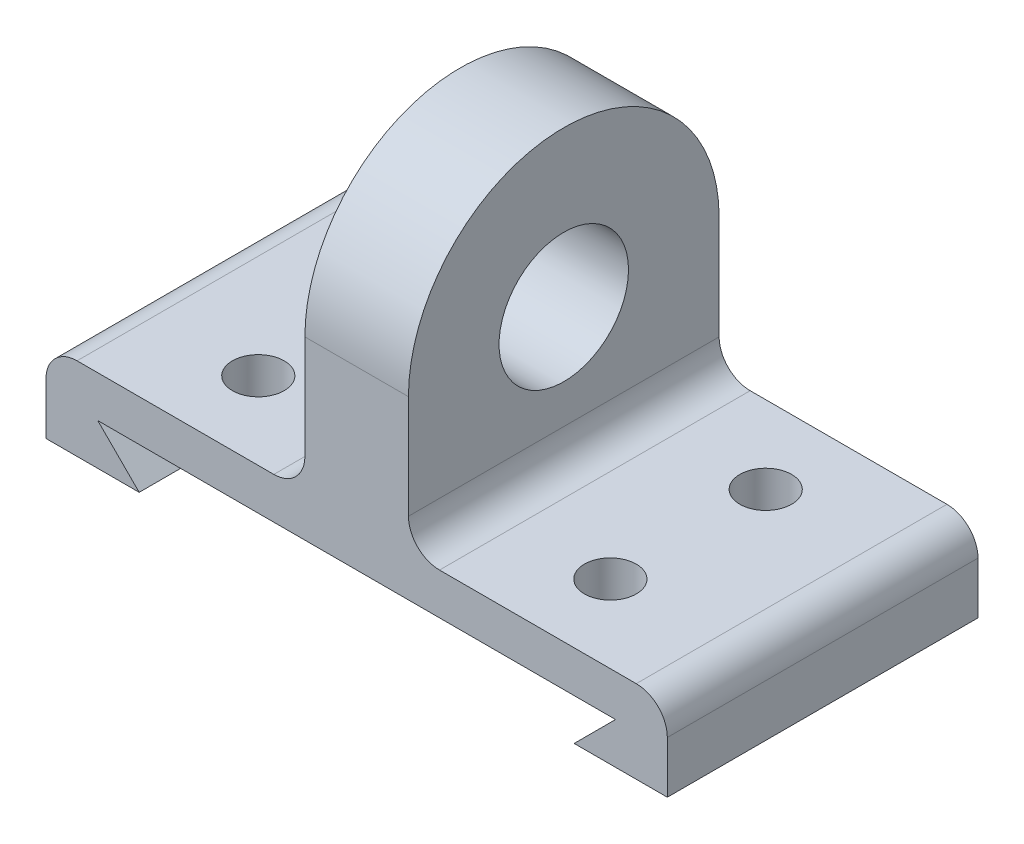
ISO-10303-21;
HEADER;
FILE_DESCRIPTION(('STEP AP214'),'2;1');
FILE_NAME('part.step','',(''),(''),'','','');
FILE_SCHEMA(('AUTOMOTIVE_DESIGN { 1 0 10303 214 1 1 1 1 }'));
ENDSEC;
DATA;
#1=APPLICATION_CONTEXT('core data for automotive mechanical design processes');
#2=APPLICATION_PROTOCOL_DEFINITION('international standard','automotive_design',2000,#1);
#3=PRODUCT_CONTEXT('',#1,'mechanical');
#4=PRODUCT('Part','Part','',(#3));
#5=PRODUCT_RELATED_PRODUCT_CATEGORY('part','',(#4));
#6=PRODUCT_DEFINITION_FORMATION('','',#4);
#7=PRODUCT_DEFINITION_CONTEXT('part definition',#1,'design');
#8=PRODUCT_DEFINITION('design','',#6,#7);
#9=PRODUCT_DEFINITION_SHAPE('','',#8);
#10=(LENGTH_UNIT() NAMED_UNIT(*) SI_UNIT(.MILLI.,.METRE.));
#11=(NAMED_UNIT(*) PLANE_ANGLE_UNIT() SI_UNIT($,.RADIAN.));
#12=(NAMED_UNIT(*) SI_UNIT($,.STERADIAN.) SOLID_ANGLE_UNIT());
#13=UNCERTAINTY_MEASURE_WITH_UNIT(LENGTH_MEASURE(1.E-05),#10,'distance_accuracy_value','');
#14=(GEOMETRIC_REPRESENTATION_CONTEXT(3) GLOBAL_UNCERTAINTY_ASSIGNED_CONTEXT((#13)) GLOBAL_UNIT_ASSIGNED_CONTEXT((#10,
#11,#12)) REPRESENTATION_CONTEXT('',''));
#15=CARTESIAN_POINT('',(0.,0.,0.));
#16=DIRECTION('',(0.,0.,1.));
#17=DIRECTION('',(1.,0.,0.));
#18=AXIS2_PLACEMENT_3D('',#15,#16,#17);
#19=CARTESIAN_POINT('',(60.,8.0000000000001,-60.));
#20=DIRECTION('',(0.,1.,0.));
#21=DIRECTION('',(-1.,0.,0.));
#22=AXIS2_PLACEMENT_3D('',#19,#20,#21);
#23=PLANE('',#22);
#24=CARTESIAN_POINT('',(-34.,8.00000000000009,-15.));
#25=DIRECTION('',(0.,1.,0.));
#26=DIRECTION('',(-1.,0.,0.));
#27=AXIS2_PLACEMENT_3D('',#24,#25,#26);
#28=CIRCLE('',#27,5.);
#29=CARTESIAN_POINT('',(-39.,8.00000000000009,-15.));
#30=VERTEX_POINT('',#29);
#31=EDGE_CURVE('E168',#30,#30,#28,.T.);
#32=ORIENTED_EDGE('',*,*,#31,.F.);
#33=EDGE_LOOP('',(#32));
#34=FACE_BOUND('',#33,.T.);
#35=CARTESIAN_POINT('',(-34.,8.00000000000009,-45.));
#36=DIRECTION('',(0.,1.,0.));
#37=DIRECTION('',(-1.,0.,0.));
#38=AXIS2_PLACEMENT_3D('',#35,#36,#37);
#39=CIRCLE('',#38,5.);
#40=CARTESIAN_POINT('',(-39.,8.00000000000009,-45.));
#41=VERTEX_POINT('',#40);
#42=EDGE_CURVE('E186',#41,#41,#39,.T.);
#43=ORIENTED_EDGE('',*,*,#42,.F.);
#44=EDGE_LOOP('',(#43));
#45=FACE_BOUND('',#44,.T.);
#46=DIRECTION('',(-1.,0.,0.));
#47=VECTOR('',#46,1.);
#48=CARTESIAN_POINT('',(60.,8.0000000000001,-60.));
#49=LINE('',#48,#47);
#50=CARTESIAN_POINT('',(-16.,8.00000000000009,-60.));
#51=VERTEX_POINT('',#50);
#52=CARTESIAN_POINT('',(-54.,8.00000000000008,-60.));
#53=VERTEX_POINT('',#52);
#54=EDGE_CURVE('E211',#51,#53,#49,.T.);
#55=ORIENTED_EDGE('',*,*,#54,.T.);
#56=DIRECTION('',(0.,0.,1.));
#57=VECTOR('',#56,1.);
#58=CARTESIAN_POINT('',(-54.,8.00000000000008,-60.));
#59=LINE('',#58,#57);
#60=CARTESIAN_POINT('',(-54.,8.00000000000008,0.));
#61=VERTEX_POINT('',#60);
#62=EDGE_CURVE('E272',#53,#61,#59,.T.);
#63=ORIENTED_EDGE('',*,*,#62,.T.);
#64=DIRECTION('',(-1.,0.,0.));
#65=VECTOR('',#64,1.);
#66=CARTESIAN_POINT('',(60.,8.0000000000001,0.));
#67=LINE('',#66,#65);
#68=CARTESIAN_POINT('',(-16.,8.00000000000009,0.));
#69=VERTEX_POINT('',#68);
#70=EDGE_CURVE('E237',#69,#61,#67,.T.);
#71=ORIENTED_EDGE('',*,*,#70,.F.);
#72=DIRECTION('',(0.,0.,-1.));
#73=VECTOR('',#72,1.);
#74=CARTESIAN_POINT('',(-16.,8.00000000000009,-60.));
#75=LINE('',#74,#73);
#76=EDGE_CURVE('E247',#69,#51,#75,.T.);
#77=ORIENTED_EDGE('',*,*,#76,.T.);
#78=EDGE_LOOP('',(#55,#63,#71,#77));
#79=FACE_BOUND('',#78,.T.);
#80=ADVANCED_FACE('F39',(#34,#45,#79),#23,.T.);
#81=CARTESIAN_POINT('',(-42.,-7.99999999999992,-60.));
#82=DIRECTION('',(0.707106781186544,0.707106781186551,0.));
#83=DIRECTION('',(-0.707106781186551,0.707106781186544,0.));
#84=AXIS2_PLACEMENT_3D('',#81,#82,#83);
#85=PLANE('',#84);
#86=DIRECTION('',(-0.707106781186551,0.707106781186544,0.));
#87=VECTOR('',#86,1.);
#88=CARTESIAN_POINT('',(-42.,-7.99999999999992,0.));
#89=LINE('',#88,#87);
#90=CARTESIAN_POINT('',(-42.,-7.99999999999992,0.));
#91=VERTEX_POINT('',#90);
#92=CARTESIAN_POINT('',(-50.,0.,0.));
#93=VERTEX_POINT('',#92);
#94=EDGE_CURVE('E201',#91,#93,#89,.T.);
#95=ORIENTED_EDGE('',*,*,#94,.F.);
#96=DIRECTION('',(0.,0.,1.));
#97=VECTOR('',#96,1.);
#98=CARTESIAN_POINT('',(-42.,-7.99999999999992,-60.));
#99=LINE('',#98,#97);
#100=CARTESIAN_POINT('',(-42.,-7.99999999999992,-60.));
#101=VERTEX_POINT('',#100);
#102=EDGE_CURVE('E253',#101,#91,#99,.T.);
#103=ORIENTED_EDGE('',*,*,#102,.F.);
#104=DIRECTION('',(-0.707106781186551,0.707106781186544,0.));
#105=VECTOR('',#104,1.);
#106=CARTESIAN_POINT('',(-42.,-7.99999999999992,-60.));
#107=LINE('',#106,#105);
#108=CARTESIAN_POINT('',(-50.,0.,-60.));
#109=VERTEX_POINT('',#108);
#110=EDGE_CURVE('E218',#101,#109,#107,.T.);
#111=ORIENTED_EDGE('',*,*,#110,.T.);
#112=DIRECTION('',(0.,0.,1.));
#113=VECTOR('',#112,1.);
#114=CARTESIAN_POINT('',(-50.,0.,-60.));
#115=LINE('',#114,#113);
#116=EDGE_CURVE('E246',#109,#93,#115,.T.);
#117=ORIENTED_EDGE('',*,*,#116,.T.);
#118=EDGE_LOOP('',(#95,#103,#111,#117));
#119=FACE_BOUND('',#118,.T.);
#120=ADVANCED_FACE('F343',(#119),#85,.T.);
#121=CARTESIAN_POINT('',(-60.,-7.99999999999992,-60.));
#122=DIRECTION('',(0.,-1.,0.));
#123=DIRECTION('',(0.,0.,-1.));
#124=AXIS2_PLACEMENT_3D('',#121,#122,#123);
#125=PLANE('',#124);
#126=DIRECTION('',(1.,0.,0.));
#127=VECTOR('',#126,1.);
#128=CARTESIAN_POINT('',(-60.,-7.99999999999992,0.));
#129=LINE('',#128,#127);
#130=CARTESIAN_POINT('',(-60.,-7.99999999999992,0.));
#131=VERTEX_POINT('',#130);
#132=EDGE_CURVE('E244',#131,#91,#129,.T.);
#133=ORIENTED_EDGE('',*,*,#132,.F.);
#134=DIRECTION('',(0.,0.,1.));
#135=VECTOR('',#134,1.);
#136=CARTESIAN_POINT('',(-60.,-7.99999999999992,-60.));
#137=LINE('',#136,#135);
#138=CARTESIAN_POINT('',(-60.,-7.99999999999992,-60.));
#139=VERTEX_POINT('',#138);
#140=EDGE_CURVE('E251',#139,#131,#137,.T.);
#141=ORIENTED_EDGE('',*,*,#140,.F.);
#142=DIRECTION('',(1.,0.,0.));
#143=VECTOR('',#142,1.);
#144=CARTESIAN_POINT('',(-60.,-7.99999999999992,-60.));
#145=LINE('',#144,#143);
#146=EDGE_CURVE('E216',#139,#101,#145,.T.);
#147=ORIENTED_EDGE('',*,*,#146,.T.);
#148=ORIENTED_EDGE('',*,*,#102,.T.);
#149=EDGE_LOOP('',(#133,#141,#147,#148));
#150=FACE_BOUND('',#149,.T.);
#151=ADVANCED_FACE('F346',(#150),#125,.T.);
#152=CARTESIAN_POINT('',(-60.,8.00000000000008,-60.));
#153=DIRECTION('',(-1.,0.,0.));
#154=DIRECTION('',(0.,0.,1.));
#155=AXIS2_PLACEMENT_3D('',#152,#153,#154);
#156=PLANE('',#155);
#157=DIRECTION('',(0.,-1.,0.));
#158=VECTOR('',#157,1.);
#159=CARTESIAN_POINT('',(-60.,8.00000000000008,0.));
#160=LINE('',#159,#158);
#161=CARTESIAN_POINT('',(-60.,2.00000000000008,0.));
#162=VERTEX_POINT('',#161);
#163=EDGE_CURVE('E238',#162,#131,#160,.T.);
#164=ORIENTED_EDGE('',*,*,#163,.F.);
#165=DIRECTION('',(0.,0.,1.));
#166=VECTOR('',#165,1.);
#167=CARTESIAN_POINT('',(-60.,2.00000000000008,-60.));
#168=LINE('',#167,#166);
#169=CARTESIAN_POINT('',(-60.,2.00000000000008,-60.));
#170=VERTEX_POINT('',#169);
#171=EDGE_CURVE('E278',#162,#170,#168,.F.);
#172=ORIENTED_EDGE('',*,*,#171,.T.);
#173=DIRECTION('',(0.,-1.,0.));
#174=VECTOR('',#173,1.);
#175=CARTESIAN_POINT('',(-60.,8.00000000000008,-60.));
#176=LINE('',#175,#174);
#177=EDGE_CURVE('E212',#170,#139,#176,.T.);
#178=ORIENTED_EDGE('',*,*,#177,.T.);
#179=ORIENTED_EDGE('',*,*,#140,.T.);
#180=EDGE_LOOP('',(#164,#172,#178,#179));
#181=FACE_BOUND('',#180,.T.);
#182=ADVANCED_FACE('F351',(#181),#156,.T.);
#183=CARTESIAN_POINT('',(54.,8.0000000000001,-60.));
#184=VERTEX_POINT('',#183);
#185=CARTESIAN_POINT('',(16.,8.00000000000009,-60.));
#186=VERTEX_POINT('',#185);
#187=EDGE_CURVE('E215',#184,#186,#49,.T.);
#188=ORIENTED_EDGE('',*,*,#187,.T.);
#189=DIRECTION('',(0.,0.,-1.));
#190=VECTOR('',#189,1.);
#191=CARTESIAN_POINT('',(16.,8.00000000000009,0.));
#192=LINE('',#191,#190);
#193=CARTESIAN_POINT('',(16.,8.00000000000009,0.));
#194=VERTEX_POINT('',#193);
#195=EDGE_CURVE('E287',#186,#194,#192,.F.);
#196=ORIENTED_EDGE('',*,*,#195,.T.);
#197=CARTESIAN_POINT('',(54.,8.0000000000001,0.));
#198=VERTEX_POINT('',#197);
#199=EDGE_CURVE('E240',#198,#194,#67,.T.);
#200=ORIENTED_EDGE('',*,*,#199,.F.);
#201=DIRECTION('',(0.,0.,1.));
#202=VECTOR('',#201,1.);
#203=CARTESIAN_POINT('',(54.,8.0000000000001,-60.));
#204=LINE('',#203,#202);
#205=EDGE_CURVE('E290',#198,#184,#204,.F.);
#206=ORIENTED_EDGE('',*,*,#205,.T.);
#207=EDGE_LOOP('',(#188,#196,#200,#206));
#208=FACE_BOUND('',#207,.T.);
#209=CARTESIAN_POINT('',(34.,8.00000000000009,-15.));
#210=DIRECTION('',(0.,1.,0.));
#211=DIRECTION('',(-1.,0.,0.));
#212=AXIS2_PLACEMENT_3D('',#209,#210,#211);
#213=CIRCLE('',#212,5.);
#214=CARTESIAN_POINT('',(29.,8.00000000000009,-15.));
#215=VERTEX_POINT('',#214);
#216=EDGE_CURVE('E194',#215,#215,#213,.T.);
#217=ORIENTED_EDGE('',*,*,#216,.F.);
#218=EDGE_LOOP('',(#217));
#219=FACE_BOUND('',#218,.T.);
#220=CARTESIAN_POINT('',(34.,8.00000000000009,-45.));
#221=DIRECTION('',(0.,1.,0.));
#222=DIRECTION('',(-1.,0.,0.));
#223=AXIS2_PLACEMENT_3D('',#220,#221,#222);
#224=CIRCLE('',#223,5.);
#225=CARTESIAN_POINT('',(29.,8.00000000000009,-45.));
#226=VERTEX_POINT('',#225);
#227=EDGE_CURVE('E193',#226,#226,#224,.T.);
#228=ORIENTED_EDGE('',*,*,#227,.F.);
#229=EDGE_LOOP('',(#228));
#230=FACE_BOUND('',#229,.T.);
#231=ADVANCED_FACE('F321',(#208,#219,#230),#23,.T.);
#232=CARTESIAN_POINT('',(60.,-7.99999999999991,-60.));
#233=DIRECTION('',(1.,0.,0.));
#234=DIRECTION('',(0.,0.,-1.));
#235=AXIS2_PLACEMENT_3D('',#232,#233,#234);
#236=PLANE('',#235);
#237=DIRECTION('',(0.,1.,0.));
#238=VECTOR('',#237,1.);
#239=CARTESIAN_POINT('',(60.,-7.99999999999991,-60.));
#240=LINE('',#239,#238);
#241=CARTESIAN_POINT('',(60.,-7.99999999999991,-60.));
#242=VERTEX_POINT('',#241);
#243=CARTESIAN_POINT('',(60.,2.0000000000001,-60.));
#244=VERTEX_POINT('',#243);
#245=EDGE_CURVE('E207',#242,#244,#240,.T.);
#246=ORIENTED_EDGE('',*,*,#245,.T.);
#247=DIRECTION('',(0.,0.,1.));
#248=VECTOR('',#247,1.);
#249=CARTESIAN_POINT('',(60.,2.0000000000001,-60.));
#250=LINE('',#249,#248);
#251=CARTESIAN_POINT('',(60.,2.0000000000001,0.));
#252=VERTEX_POINT('',#251);
#253=EDGE_CURVE('E295',#244,#252,#250,.T.);
#254=ORIENTED_EDGE('',*,*,#253,.T.);
#255=DIRECTION('',(0.,1.,0.));
#256=VECTOR('',#255,1.);
#257=CARTESIAN_POINT('',(60.,-7.99999999999991,0.));
#258=LINE('',#257,#256);
#259=CARTESIAN_POINT('',(60.,-7.99999999999991,0.));
#260=VERTEX_POINT('',#259);
#261=EDGE_CURVE('E235',#260,#252,#258,.T.);
#262=ORIENTED_EDGE('',*,*,#261,.F.);
#263=DIRECTION('',(0.,0.,1.));
#264=VECTOR('',#263,1.);
#265=CARTESIAN_POINT('',(60.,-7.99999999999991,-60.));
#266=LINE('',#265,#264);
#267=EDGE_CURVE('E258',#242,#260,#266,.T.);
#268=ORIENTED_EDGE('',*,*,#267,.F.);
#269=EDGE_LOOP('',(#246,#254,#262,#268));
#270=FACE_BOUND('',#269,.T.);
#271=ADVANCED_FACE('F327',(#270),#236,.T.);
#272=CARTESIAN_POINT('',(42.,-7.99999999999991,-60.));
#273=DIRECTION('',(0.,-1.,0.));
#274=DIRECTION('',(0.,0.,-1.));
#275=AXIS2_PLACEMENT_3D('',#272,#273,#274);
#276=PLANE('',#275);
#277=DIRECTION('',(1.,0.,0.));
#278=VECTOR('',#277,1.);
#279=CARTESIAN_POINT('',(42.,-7.99999999999991,0.));
#280=LINE('',#279,#278);
#281=CARTESIAN_POINT('',(42.,-7.99999999999991,0.));
#282=VERTEX_POINT('',#281);
#283=EDGE_CURVE('E226',#282,#260,#280,.T.);
#284=ORIENTED_EDGE('',*,*,#283,.F.);
#285=DIRECTION('',(0.,0.,1.));
#286=VECTOR('',#285,1.);
#287=CARTESIAN_POINT('',(42.,-7.99999999999991,-60.));
#288=LINE('',#287,#286);
#289=CARTESIAN_POINT('',(42.,-7.99999999999991,-60.));
#290=VERTEX_POINT('',#289);
#291=EDGE_CURVE('E256',#290,#282,#288,.T.);
#292=ORIENTED_EDGE('',*,*,#291,.F.);
#293=DIRECTION('',(1.,0.,0.));
#294=VECTOR('',#293,1.);
#295=CARTESIAN_POINT('',(42.,-7.99999999999991,-60.));
#296=LINE('',#295,#294);
#297=EDGE_CURVE('E206',#290,#242,#296,.T.);
#298=ORIENTED_EDGE('',*,*,#297,.T.);
#299=ORIENTED_EDGE('',*,*,#267,.T.);
#300=EDGE_LOOP('',(#284,#292,#298,#299));
#301=FACE_BOUND('',#300,.T.);
#302=ADVANCED_FACE('F334',(#301),#276,.T.);
#303=CARTESIAN_POINT('',(50.,0.,-60.));
#304=DIRECTION('',(-0.707106781186544,0.707106781186551,0.));
#305=DIRECTION('',(-0.707106781186551,-0.707106781186544,0.));
#306=AXIS2_PLACEMENT_3D('',#303,#304,#305);
#307=PLANE('',#306);
#308=DIRECTION('',(-0.707106781186551,-0.707106781186544,0.));
#309=VECTOR('',#308,1.);
#310=CARTESIAN_POINT('',(50.,0.,0.));
#311=LINE('',#310,#309);
#312=CARTESIAN_POINT('',(50.,0.,0.));
#313=VERTEX_POINT('',#312);
#314=EDGE_CURVE('E228',#313,#282,#311,.T.);
#315=ORIENTED_EDGE('',*,*,#314,.F.);
#316=DIRECTION('',(0.,0.,1.));
#317=VECTOR('',#316,1.);
#318=CARTESIAN_POINT('',(50.,0.,-60.));
#319=LINE('',#318,#317);
#320=CARTESIAN_POINT('',(50.,0.,-60.));
#321=VERTEX_POINT('',#320);
#322=EDGE_CURVE('E225',#321,#313,#319,.T.);
#323=ORIENTED_EDGE('',*,*,#322,.F.);
#324=DIRECTION('',(-0.707106781186551,-0.707106781186544,0.));
#325=VECTOR('',#324,1.);
#326=CARTESIAN_POINT('',(50.,0.,-60.));
#327=LINE('',#326,#325);
#328=EDGE_CURVE('E205',#321,#290,#327,.T.);
#329=ORIENTED_EDGE('',*,*,#328,.T.);
#330=ORIENTED_EDGE('',*,*,#291,.T.);
#331=EDGE_LOOP('',(#315,#323,#329,#330));
#332=FACE_BOUND('',#331,.T.);
#333=ADVANCED_FACE('F338',(#332),#307,.T.);
#334=CARTESIAN_POINT('',(0.,0.,-60.));
#335=DIRECTION('',(0.,-1.,0.));
#336=DIRECTION('',(0.,0.,-1.));
#337=AXIS2_PLACEMENT_3D('',#334,#335,#336);
#338=PLANE('',#337);
#339=CARTESIAN_POINT('',(34.,0.,-15.));
#340=DIRECTION('',(0.,-1.,0.));
#341=DIRECTION('',(0.,0.,-1.));
#342=AXIS2_PLACEMENT_3D('',#339,#340,#341);
#343=CIRCLE('',#342,5.);
#344=CARTESIAN_POINT('',(34.,0.,-20.));
#345=VERTEX_POINT('',#344);
#346=EDGE_CURVE('E229',#345,#345,#343,.T.);
#347=ORIENTED_EDGE('',*,*,#346,.F.);
#348=EDGE_LOOP('',(#347));
#349=FACE_BOUND('',#348,.T.);
#350=CARTESIAN_POINT('',(-34.,0.,-45.));
#351=DIRECTION('',(0.,-1.,0.));
#352=DIRECTION('',(0.,0.,-1.));
#353=AXIS2_PLACEMENT_3D('',#350,#351,#352);
#354=CIRCLE('',#353,5.);
#355=CARTESIAN_POINT('',(-34.,0.,-50.));
#356=VERTEX_POINT('',#355);
#357=EDGE_CURVE('E266',#356,#356,#354,.T.);
#358=ORIENTED_EDGE('',*,*,#357,.F.);
#359=EDGE_LOOP('',(#358));
#360=FACE_BOUND('',#359,.T.);
#361=CARTESIAN_POINT('',(-34.,0.,-15.));
#362=DIRECTION('',(0.,-1.,0.));
#363=DIRECTION('',(0.,0.,-1.));
#364=AXIS2_PLACEMENT_3D('',#361,#362,#363);
#365=CIRCLE('',#364,5.);
#366=CARTESIAN_POINT('',(-34.,0.,-20.));
#367=VERTEX_POINT('',#366);
#368=EDGE_CURVE('E263',#367,#367,#365,.T.);
#369=ORIENTED_EDGE('',*,*,#368,.F.);
#370=EDGE_LOOP('',(#369));
#371=FACE_BOUND('',#370,.T.);
#372=CARTESIAN_POINT('',(34.,0.,-45.));
#373=DIRECTION('',(0.,-1.,0.));
#374=DIRECTION('',(0.,0.,-1.));
#375=AXIS2_PLACEMENT_3D('',#372,#373,#374);
#376=CIRCLE('',#375,5.);
#377=CARTESIAN_POINT('',(34.,0.,-50.));
#378=VERTEX_POINT('',#377);
#379=EDGE_CURVE('E200',#378,#378,#376,.T.);
#380=ORIENTED_EDGE('',*,*,#379,.F.);
#381=EDGE_LOOP('',(#380));
#382=FACE_BOUND('',#381,.T.);
#383=DIRECTION('',(1.,0.,0.));
#384=VECTOR('',#383,1.);
#385=CARTESIAN_POINT('',(0.,0.,0.));
#386=LINE('',#385,#384);
#387=EDGE_CURVE('E224',#93,#313,#386,.T.);
#388=ORIENTED_EDGE('',*,*,#387,.F.);
#389=ORIENTED_EDGE('',*,*,#116,.F.);
#390=DIRECTION('',(1.,0.,0.));
#391=VECTOR('',#390,1.);
#392=CARTESIAN_POINT('',(-50.,0.,-60.));
#393=LINE('',#392,#391);
#394=EDGE_CURVE('E199',#109,#321,#393,.T.);
#395=ORIENTED_EDGE('',*,*,#394,.T.);
#396=ORIENTED_EDGE('',*,*,#322,.T.);
#397=EDGE_LOOP('',(#388,#389,#395,#396));
#398=FACE_BOUND('',#397,.T.);
#399=ADVANCED_FACE('F359',(#349,#360,#371,#382,#398),#338,.T.);
#400=CARTESIAN_POINT('',(0.,0.,-60.));
#401=DIRECTION('',(0.,0.,1.));
#402=DIRECTION('',(1.,0.,0.));
#403=AXIS2_PLACEMENT_3D('',#400,#401,#402);
#404=PLANE('',#403);
#405=ORIENTED_EDGE('',*,*,#177,.F.);
#406=CARTESIAN_POINT('',(-54.,2.00000000000008,-60.));
#407=DIRECTION('',(0.,0.,1.));
#408=DIRECTION('',(1.,0.,0.));
#409=AXIS2_PLACEMENT_3D('',#406,#407,#408);
#410=CIRCLE('',#409,6.);
#411=EDGE_CURVE('E282',#170,#53,#410,.F.);
#412=ORIENTED_EDGE('',*,*,#411,.T.);
#413=ORIENTED_EDGE('',*,*,#54,.F.);
#414=CARTESIAN_POINT('',(-16.,14.0000000000001,-60.));
#415=DIRECTION('',(0.,0.,1.));
#416=DIRECTION('',(1.,0.,0.));
#417=AXIS2_PLACEMENT_3D('',#414,#415,#416);
#418=CIRCLE('',#417,6.);
#419=CARTESIAN_POINT('',(-10.,14.0000000000001,-60.));
#420=VERTEX_POINT('',#419);
#421=EDGE_CURVE('E293',#51,#420,#418,.T.);
#422=ORIENTED_EDGE('',*,*,#421,.T.);
#423=DIRECTION('',(0.,1.,0.));
#424=VECTOR('',#423,1.);
#425=CARTESIAN_POINT('',(-10.,8.0000000000001,-60.));
#426=LINE('',#425,#424);
#427=CARTESIAN_POINT('',(-10.,34.0000000000001,-60.));
#428=VERTEX_POINT('',#427);
#429=EDGE_CURVE('E170',#420,#428,#426,.T.);
#430=ORIENTED_EDGE('',*,*,#429,.T.);
#431=DIRECTION('',(-1.,0.,0.));
#432=VECTOR('',#431,1.);
#433=CARTESIAN_POINT('',(10.,34.0000000000001,-60.));
#434=LINE('',#433,#432);
#435=CARTESIAN_POINT('',(10.,34.0000000000001,-60.));
#436=VERTEX_POINT('',#435);
#437=EDGE_CURVE('E162',#436,#428,#434,.T.);
#438=ORIENTED_EDGE('',*,*,#437,.F.);
#439=DIRECTION('',(0.,1.,0.));
#440=VECTOR('',#439,1.);
#441=CARTESIAN_POINT('',(10.,8.0000000000001,-60.));
#442=LINE('',#441,#440);
#443=CARTESIAN_POINT('',(10.,14.0000000000001,-60.));
#444=VERTEX_POINT('',#443);
#445=EDGE_CURVE('E147',#444,#436,#442,.T.);
#446=ORIENTED_EDGE('',*,*,#445,.F.);
#447=CARTESIAN_POINT('',(16.,14.0000000000001,-60.));
#448=DIRECTION('',(0.,0.,1.));
#449=DIRECTION('',(1.,0.,0.));
#450=AXIS2_PLACEMENT_3D('',#447,#448,#449);
#451=CIRCLE('',#450,6.);
#452=EDGE_CURVE('E50',#444,#186,#451,.T.);
#453=ORIENTED_EDGE('',*,*,#452,.T.);
#454=ORIENTED_EDGE('',*,*,#187,.F.);
#455=CARTESIAN_POINT('',(54.,2.0000000000001,-60.));
#456=DIRECTION('',(0.,0.,1.));
#457=DIRECTION('',(1.,0.,0.));
#458=AXIS2_PLACEMENT_3D('',#455,#456,#457);
#459=CIRCLE('',#458,6.);
#460=EDGE_CURVE('E53',#184,#244,#459,.F.);
#461=ORIENTED_EDGE('',*,*,#460,.T.);
#462=ORIENTED_EDGE('',*,*,#245,.F.);
#463=ORIENTED_EDGE('',*,*,#297,.F.);
#464=ORIENTED_EDGE('',*,*,#328,.F.);
#465=ORIENTED_EDGE('',*,*,#394,.F.);
#466=ORIENTED_EDGE('',*,*,#110,.F.);
#467=ORIENTED_EDGE('',*,*,#146,.F.);
#468=EDGE_LOOP('',(#405,#412,#413,#422,#430,#438,#446,#453,#454,#461,#462,#463,#464,#465,#466,#467));
#469=FACE_BOUND('',#468,.T.);
#470=ADVANCED_FACE('F164',(#469),#404,.F.);
#471=CARTESIAN_POINT('',(0.,0.,0.));
#472=DIRECTION('',(0.,0.,1.));
#473=DIRECTION('',(1.,0.,0.));
#474=AXIS2_PLACEMENT_3D('',#471,#472,#473);
#475=PLANE('',#474);
#476=ORIENTED_EDGE('',*,*,#70,.T.);
#477=CARTESIAN_POINT('',(-54.,2.00000000000008,0.));
#478=DIRECTION('',(0.,0.,1.));
#479=DIRECTION('',(1.,0.,0.));
#480=AXIS2_PLACEMENT_3D('',#477,#478,#479);
#481=CIRCLE('',#480,6.);
#482=EDGE_CURVE('E279',#61,#162,#481,.T.);
#483=ORIENTED_EDGE('',*,*,#482,.T.);
#484=ORIENTED_EDGE('',*,*,#163,.T.);
#485=ORIENTED_EDGE('',*,*,#132,.T.);
#486=ORIENTED_EDGE('',*,*,#94,.T.);
#487=ORIENTED_EDGE('',*,*,#387,.T.);
#488=ORIENTED_EDGE('',*,*,#314,.T.);
#489=ORIENTED_EDGE('',*,*,#283,.T.);
#490=ORIENTED_EDGE('',*,*,#261,.T.);
#491=CARTESIAN_POINT('',(54.,2.0000000000001,0.));
#492=DIRECTION('',(0.,0.,1.));
#493=DIRECTION('',(1.,0.,0.));
#494=AXIS2_PLACEMENT_3D('',#491,#492,#493);
#495=CIRCLE('',#494,6.);
#496=EDGE_CURVE('E277',#252,#198,#495,.T.);
#497=ORIENTED_EDGE('',*,*,#496,.T.);
#498=ORIENTED_EDGE('',*,*,#199,.T.);
#499=CARTESIAN_POINT('',(16.,14.0000000000001,0.));
#500=DIRECTION('',(0.,0.,1.));
#501=DIRECTION('',(1.,0.,0.));
#502=AXIS2_PLACEMENT_3D('',#499,#500,#501);
#503=CIRCLE('',#502,6.);
#504=CARTESIAN_POINT('',(10.,14.0000000000001,0.));
#505=VERTEX_POINT('',#504);
#506=EDGE_CURVE('E11',#194,#505,#503,.F.);
#507=ORIENTED_EDGE('',*,*,#506,.T.);
#508=DIRECTION('',(0.,-1.,0.));
#509=VECTOR('',#508,1.);
#510=CARTESIAN_POINT('',(10.,8.0000000000001,0.));
#511=LINE('',#510,#509);
#512=CARTESIAN_POINT('',(10.,34.0000000000001,0.));
#513=VERTEX_POINT('',#512);
#514=EDGE_CURVE('E179',#513,#505,#511,.T.);
#515=ORIENTED_EDGE('',*,*,#514,.F.);
#516=DIRECTION('',(-1.,0.,0.));
#517=VECTOR('',#516,1.);
#518=CARTESIAN_POINT('',(10.,34.0000000000001,0.));
#519=LINE('',#518,#517);
#520=CARTESIAN_POINT('',(-10.,34.0000000000001,0.));
#521=VERTEX_POINT('',#520);
#522=EDGE_CURVE('E173',#513,#521,#519,.T.);
#523=ORIENTED_EDGE('',*,*,#522,.T.);
#524=DIRECTION('',(0.,-1.,0.));
#525=VECTOR('',#524,1.);
#526=CARTESIAN_POINT('',(-10.,8.0000000000001,0.));
#527=LINE('',#526,#525);
#528=CARTESIAN_POINT('',(-10.,14.0000000000001,0.));
#529=VERTEX_POINT('',#528);
#530=EDGE_CURVE('E159',#521,#529,#527,.T.);
#531=ORIENTED_EDGE('',*,*,#530,.T.);
#532=CARTESIAN_POINT('',(-16.,14.0000000000001,0.));
#533=DIRECTION('',(0.,0.,1.));
#534=DIRECTION('',(1.,0.,0.));
#535=AXIS2_PLACEMENT_3D('',#532,#533,#534);
#536=CIRCLE('',#535,6.);
#537=EDGE_CURVE('E299',#529,#69,#536,.F.);
#538=ORIENTED_EDGE('',*,*,#537,.T.);
#539=EDGE_LOOP('',(#476,#483,#484,#485,#486,#487,#488,#489,#490,#497,#498,#507,#515,#523,#531,#538));
#540=FACE_BOUND('',#539,.T.);
#541=ADVANCED_FACE('F301',(#540),#475,.T.);
#542=CARTESIAN_POINT('',(34.,-51.9999999999999,-45.));
#543=DIRECTION('',(0.,1.,0.));
#544=DIRECTION('',(-1.,0.,0.));
#545=AXIS2_PLACEMENT_3D('',#542,#543,#544);
#546=CYLINDRICAL_SURFACE('',#545,5.);
#547=ORIENTED_EDGE('',*,*,#379,.T.);
#548=EDGE_LOOP('',(#547));
#549=FACE_BOUND('',#548,.T.);
#550=ORIENTED_EDGE('',*,*,#227,.T.);
#551=EDGE_LOOP('',(#550));
#552=FACE_BOUND('',#551,.T.);
#553=ADVANCED_FACE('F392',(#549,#552),#546,.F.);
#554=CARTESIAN_POINT('',(-34.,-51.9999999999999,-15.));
#555=DIRECTION('',(0.,1.,0.));
#556=DIRECTION('',(-1.,0.,0.));
#557=AXIS2_PLACEMENT_3D('',#554,#555,#556);
#558=CYLINDRICAL_SURFACE('',#557,5.);
#559=ORIENTED_EDGE('',*,*,#368,.T.);
#560=EDGE_LOOP('',(#559));
#561=FACE_BOUND('',#560,.T.);
#562=ORIENTED_EDGE('',*,*,#31,.T.);
#563=EDGE_LOOP('',(#562));
#564=FACE_BOUND('',#563,.T.);
#565=ADVANCED_FACE('F399',(#561,#564),#558,.F.);
#566=CARTESIAN_POINT('',(-34.,-51.9999999999999,-45.));
#567=DIRECTION('',(0.,1.,0.));
#568=DIRECTION('',(-1.,0.,0.));
#569=AXIS2_PLACEMENT_3D('',#566,#567,#568);
#570=CYLINDRICAL_SURFACE('',#569,5.);
#571=ORIENTED_EDGE('',*,*,#357,.T.);
#572=EDGE_LOOP('',(#571));
#573=FACE_BOUND('',#572,.T.);
#574=ORIENTED_EDGE('',*,*,#42,.T.);
#575=EDGE_LOOP('',(#574));
#576=FACE_BOUND('',#575,.T.);
#577=ADVANCED_FACE('F400',(#573,#576),#570,.F.);
#578=CARTESIAN_POINT('',(34.,-51.9999999999999,-15.));
#579=DIRECTION('',(0.,1.,0.));
#580=DIRECTION('',(-1.,0.,0.));
#581=AXIS2_PLACEMENT_3D('',#578,#579,#580);
#582=CYLINDRICAL_SURFACE('',#581,5.);
#583=ORIENTED_EDGE('',*,*,#346,.T.);
#584=EDGE_LOOP('',(#583));
#585=FACE_BOUND('',#584,.T.);
#586=ORIENTED_EDGE('',*,*,#216,.T.);
#587=EDGE_LOOP('',(#586));
#588=FACE_BOUND('',#587,.T.);
#589=ADVANCED_FACE('F402',(#585,#588),#582,.F.);
#590=CARTESIAN_POINT('',(10.,34.0000000000001,-30.));
#591=DIRECTION('',(1.,0.,0.));
#592=DIRECTION('',(0.,0.,-1.));
#593=AXIS2_PLACEMENT_3D('',#590,#591,#592);
#594=PLANE('',#593);
#595=ORIENTED_EDGE('',*,*,#514,.T.);
#596=DIRECTION('',(0.,0.,-1.));
#597=VECTOR('',#596,1.);
#598=CARTESIAN_POINT('',(10.,14.0000000000001,-60.));
#599=LINE('',#598,#597);
#600=EDGE_CURVE('E157',#505,#444,#599,.T.);
#601=ORIENTED_EDGE('',*,*,#600,.T.);
#602=ORIENTED_EDGE('',*,*,#445,.T.);
#603=CARTESIAN_POINT('',(10.,34.0000000000001,-30.));
#604=DIRECTION('',(1.,0.,0.));
#605=DIRECTION('',(0.,0.,-1.));
#606=AXIS2_PLACEMENT_3D('',#603,#604,#605);
#607=CIRCLE('',#606,30.);
#608=EDGE_CURVE('E156',#436,#513,#607,.T.);
#609=ORIENTED_EDGE('',*,*,#608,.T.);
#610=EDGE_LOOP('',(#595,#601,#602,#609));
#611=FACE_BOUND('',#610,.T.);
#612=CARTESIAN_POINT('',(10.,34.0000000000001,-30.));
#613=DIRECTION('',(1.,0.,0.));
#614=DIRECTION('',(0.,0.,-1.));
#615=AXIS2_PLACEMENT_3D('',#612,#613,#614);
#616=CIRCLE('',#615,12.5);
#617=CARTESIAN_POINT('',(10.,34.0000000000001,-42.5));
#618=VERTEX_POINT('',#617);
#619=EDGE_CURVE('E181',#618,#618,#616,.T.);
#620=ORIENTED_EDGE('',*,*,#619,.F.);
#621=EDGE_LOOP('',(#620));
#622=FACE_BOUND('',#621,.T.);
#623=ADVANCED_FACE('F153',(#611,#622),#594,.T.);
#624=CARTESIAN_POINT('',(-10.,34.0000000000001,-30.));
#625=DIRECTION('',(1.,0.,0.));
#626=DIRECTION('',(0.,0.,-1.));
#627=AXIS2_PLACEMENT_3D('',#624,#625,#626);
#628=PLANE('',#627);
#629=ORIENTED_EDGE('',*,*,#429,.F.);
#630=DIRECTION('',(0.,0.,-1.));
#631=VECTOR('',#630,1.);
#632=CARTESIAN_POINT('',(-10.,14.0000000000001,-30.));
#633=LINE('',#632,#631);
#634=EDGE_CURVE('E281',#420,#529,#633,.F.);
#635=ORIENTED_EDGE('',*,*,#634,.T.);
#636=ORIENTED_EDGE('',*,*,#530,.F.);
#637=CARTESIAN_POINT('',(-10.,34.0000000000001,-30.));
#638=DIRECTION('',(1.,0.,0.));
#639=DIRECTION('',(0.,0.,-1.));
#640=AXIS2_PLACEMENT_3D('',#637,#638,#639);
#641=CIRCLE('',#640,30.);
#642=EDGE_CURVE('E185',#428,#521,#641,.T.);
#643=ORIENTED_EDGE('',*,*,#642,.F.);
#644=EDGE_LOOP('',(#629,#635,#636,#643));
#645=FACE_BOUND('',#644,.T.);
#646=CARTESIAN_POINT('',(-10.,34.0000000000001,-30.));
#647=DIRECTION('',(1.,0.,0.));
#648=DIRECTION('',(0.,0.,-1.));
#649=AXIS2_PLACEMENT_3D('',#646,#647,#648);
#650=CIRCLE('',#649,12.5);
#651=CARTESIAN_POINT('',(-10.,34.0000000000001,-42.5));
#652=VERTEX_POINT('',#651);
#653=EDGE_CURVE('E422',#652,#652,#650,.T.);
#654=ORIENTED_EDGE('',*,*,#653,.T.);
#655=EDGE_LOOP('',(#654));
#656=FACE_BOUND('',#655,.T.);
#657=ADVANCED_FACE('F311',(#645,#656),#628,.F.);
#658=CARTESIAN_POINT('',(10.,34.0000000000001,-30.));
#659=DIRECTION('',(-1.,0.,0.));
#660=DIRECTION('',(0.,0.,1.));
#661=AXIS2_PLACEMENT_3D('',#658,#659,#660);
#662=CYLINDRICAL_SURFACE('',#661,30.);
#663=ORIENTED_EDGE('',*,*,#642,.T.);
#664=ORIENTED_EDGE('',*,*,#522,.F.);
#665=ORIENTED_EDGE('',*,*,#608,.F.);
#666=ORIENTED_EDGE('',*,*,#437,.T.);
#667=EDGE_LOOP('',(#663,#664,#665,#666));
#668=FACE_BOUND('',#667,.T.);
#669=ADVANCED_FACE('F172',(#668),#662,.T.);
#670=CARTESIAN_POINT('',(10.,34.0000000000001,-30.));
#671=DIRECTION('',(-1.,0.,0.));
#672=DIRECTION('',(0.,0.,1.));
#673=AXIS2_PLACEMENT_3D('',#670,#671,#672);
#674=CYLINDRICAL_SURFACE('',#673,12.5);
#675=ORIENTED_EDGE('',*,*,#619,.T.);
#676=EDGE_LOOP('',(#675));
#677=FACE_BOUND('',#676,.T.);
#678=ORIENTED_EDGE('',*,*,#653,.F.);
#679=EDGE_LOOP('',(#678));
#680=FACE_BOUND('',#679,.T.);
#681=ADVANCED_FACE('F414',(#677,#680),#674,.F.);
#682=CARTESIAN_POINT('',(-54.,2.00000000000008,-60.));
#683=DIRECTION('',(0.,0.,1.));
#684=DIRECTION('',(1.,0.,0.));
#685=AXIS2_PLACEMENT_3D('',#682,#683,#684);
#686=CYLINDRICAL_SURFACE('',#685,6.);
#687=ORIENTED_EDGE('',*,*,#411,.F.);
#688=ORIENTED_EDGE('',*,*,#171,.F.);
#689=ORIENTED_EDGE('',*,*,#482,.F.);
#690=ORIENTED_EDGE('',*,*,#62,.F.);
#691=EDGE_LOOP('',(#687,#688,#689,#690));
#692=FACE_BOUND('',#691,.T.);
#693=ADVANCED_FACE('F352',(#692),#686,.T.);
#694=CARTESIAN_POINT('',(-16.,14.0000000000001,-60.));
#695=DIRECTION('',(0.,0.,-1.));
#696=DIRECTION('',(-1.,0.,0.));
#697=AXIS2_PLACEMENT_3D('',#694,#695,#696);
#698=CYLINDRICAL_SURFACE('',#697,6.);
#699=ORIENTED_EDGE('',*,*,#537,.F.);
#700=ORIENTED_EDGE('',*,*,#634,.F.);
#701=ORIENTED_EDGE('',*,*,#421,.F.);
#702=ORIENTED_EDGE('',*,*,#76,.F.);
#703=EDGE_LOOP('',(#699,#700,#701,#702));
#704=FACE_BOUND('',#703,.T.);
#705=ADVANCED_FACE('F313',(#704),#698,.F.);
#706=CARTESIAN_POINT('',(16.,14.0000000000001,-30.));
#707=DIRECTION('',(0.,0.,1.));
#708=DIRECTION('',(1.,0.,0.));
#709=AXIS2_PLACEMENT_3D('',#706,#707,#708);
#710=CYLINDRICAL_SURFACE('',#709,6.);
#711=ORIENTED_EDGE('',*,*,#506,.F.);
#712=ORIENTED_EDGE('',*,*,#195,.F.);
#713=ORIENTED_EDGE('',*,*,#452,.F.);
#714=ORIENTED_EDGE('',*,*,#600,.F.);
#715=EDGE_LOOP('',(#711,#712,#713,#714));
#716=FACE_BOUND('',#715,.T.);
#717=ADVANCED_FACE('F320',(#716),#710,.F.);
#718=CARTESIAN_POINT('',(54.,2.0000000000001,-60.));
#719=DIRECTION('',(0.,0.,1.));
#720=DIRECTION('',(1.,0.,0.));
#721=AXIS2_PLACEMENT_3D('',#718,#719,#720);
#722=CYLINDRICAL_SURFACE('',#721,6.);
#723=ORIENTED_EDGE('',*,*,#460,.F.);
#724=ORIENTED_EDGE('',*,*,#205,.F.);
#725=ORIENTED_EDGE('',*,*,#496,.F.);
#726=ORIENTED_EDGE('',*,*,#253,.F.);
#727=EDGE_LOOP('',(#723,#724,#725,#726));
#728=FACE_BOUND('',#727,.T.);
#729=ADVANCED_FACE('F41',(#728),#722,.T.);
#730=CLOSED_SHELL('',(#80,#120,#151,#182,#231,#271,#302,#333,#399,#470,#541,#553,#565,#577,#589,
#623,#657,#669,#681,#693,#705,#717,#729));
#731=MANIFOLD_SOLID_BREP('B2',#730);
#732=ADVANCED_BREP_SHAPE_REPRESENTATION('',(#18,#731),#14);
#733=SHAPE_DEFINITION_REPRESENTATION(#9,#732);
ENDSEC;
END-ISO-10303-21;
